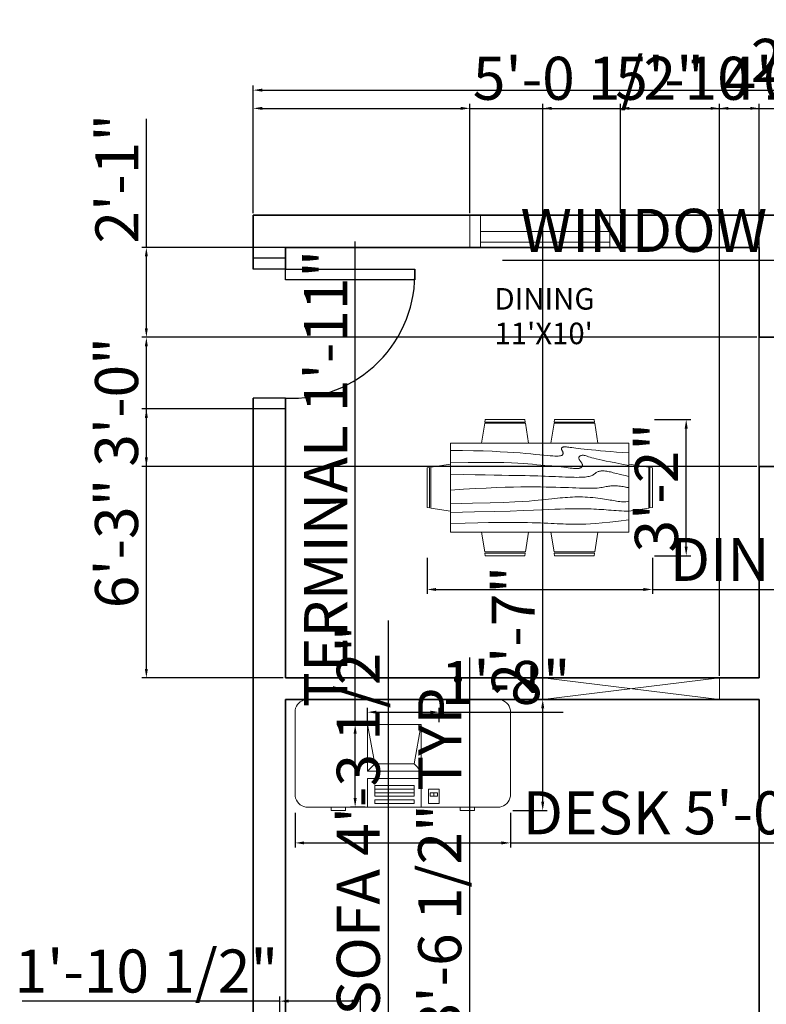
# Model space of a CAD drawing. Units: inches. Extents: x 2011 to 2548, y 530 to 1188.
# Tile 3 of 5: x 2011 to 2220, y 891 to 1166. Entities that reach past the tile are written whole.
import ezdxf

# ---------------------------------------------------------------- set-up
doc = ezdxf.new("R2010")
doc.units = ezdxf.units.IN
for name, color, linetype, lineweight in [('A-ANNO-DIMS', 2, 'Continuous', 18), ('A-AREA-IDEN', 7, 'Continuous', 25), ('A-DOOR', 3, 'Continuous', 25), ('A-EQPM', 8, 'Continuous', 18), ('A-FURN', 8, 'Continuous', 18), ('A-GLAZ', 4, 'Continuous', 18), ('A-WALL', 7, 'Continuous', 35), ('A-WALL-OPEN', 4, 'Continuous', 18)]:
    doc.layers.add(name, color=color, linetype=linetype, lineweight=lineweight)
doc.styles.get("Standard").update_dxf_attribs({"font": 'arial.ttf'})
doc.dimstyles.new('ISO-25', dxfattribs={"dimtxt": 12, "dimasz": 2.5, "dimexe": 1.25, "dimexo": 0.625, "dimtad": 1, "dimdec": 1, "dimlunit": 3, "dimtxsty": 'Standard', "dimcen": 2.5, "dimadec": 0, "dimazin": 0, "dimtfac": 1, "dimtdec": 1, "dimtmove": 0, "dimatfit": 3, "dimfxl": 1, "dimarcsym": 0})

# ---------------------------------------------------------------- blocks, each defined once
blk = doc.blocks.new('Desk - 30 x 60 in.')
for p, q in [((-26.999995, 0), (26.999995, 0)), ((-29.999995, -27), (-29.999995, -3)), ((29.999995, -3), (29.999995, -27)), ((26.999995, -30), (-26.999995, -30)), ((-20.000005, -30), (-20.000005, -31)), ((-16.000005, -31), (-16.000005, -30)), ((15.999995, -31), (15.999995, -30)), ((19.999995, -30), (19.999995, -31)), ((-20.000005, -31), (-16.000005, -31)), ((19.999995, -31), (15.999995, -31))]:
    blk.add_line(p, q)
for centre, start, end in [((-26.499995, -3.5), 98.1301, 171.8699), ((26.499995, -3.5), 8.130102, 81.8699), ((-26.499995, -26.5), 188.1301, 261.8699), ((26.499995, -26.5), 278.1301, 351.8699)]:
    blk.add_arc(centre, 3.535534, start, end)
blk = doc.blocks.new('Computer Terminal')
for p, q in [((-10, 11.5), (5, 11.5)), ((-8, 0.5), (-10, 11.5)), ((-10, -1.5), (-10, 11.5)), ((5, 11.5), (3, 0.5)), ((5, 11.5), (5, -1.5)), ((-10, -1.5), (-8, 0.5)), ((3, 0.5), (-8, 0.5)), ((3, 0.5), (5, -1.5)), ((5, -1.5), (-10, -1.5)), ((-10, -11.5), (-10, -3.5)), ((-10, -3.5), (5, -3.5)), ((5, -3.5), (5, -11.5)), ((-8, -5.5), (-8, -8.5)), ((3, -5.5), (-8, -5.5)), ((3, -6.5), (-8, -6.5)), ((-8, -7.5), (3, -7.5)), ((3, -8.5), (3, -5.5)), ((10, -6.5), (7, -6.5)), ((7, -6.5), (7, -10.5)), ((9.5, -7.5), (7.5, -7.5)), ((7.5, -7.5), (7.5, -8.5)), ((8.5, -7.5), (8.5, -8.5)), ((9.5, -8.5), (9.5, -7.5)), ((10, -10.5), (10, -6.5)), ((-8, -8.5), (3, -8.5)), ((-8, -9.5), (-8, -10.5)), ((3, -9.5), (-8, -9.5)), ((-8, -10.5), (3, -10.5)), ((3, -10.5), (3, -9.5)), ((7, -10.5), (10, -10.5)), ((7.5, -8.5), (9.5, -8.5)), ((5, -11.5), (-10, -11.5))]:
    blk.add_line(p, q)
blk = doc.blocks.new('Dining Set - 36 x 72 in.')
for p, q in [((-22.2343, 26.00059), (-23.4847, 17.99762)), ((-22.2304, 26), (-5.7608, 26)), ((-22, 27.5), (-22.1562, 26.50042)), ((-5.8416, 26.5), (-22.1534, 26.5)), ((-22, 27.5), (-6, 27.5)), ((-5.8437, 26.49966), (-6, 27.5)), ((-4.5152, 17.99762), (-5.7655, 25.99926)), ((5.7657, 26.00059), (4.5153, 17.99762)), ((5.7696, 26), (22.2392, 26)), ((6, 27.5), (5.8438, 26.50042)), ((22.1584, 26.5), (5.8466, 26.5)), ((6, 27.5), (22, 27.5)), ((22.1563, 26.49966), (22, 27.5)), ((23.4848, 17.99762), (22.2345, 25.99926)), ((36, 18), (-36, 18)), ((-36, 18), (-36, -18)), ((36, -18), (36, 18)), ((-45.5, 8), (-44.5004, 8.15617)), ((-45.5, 8), (-45.5, -8)), ((-44.5, -8.15843), (-44.5, 8.15338)), ((-44.0006, 8.23428), (-35.9976, 9.48474)), ((-44, 8.23041), (-44, -8.23915)), ((44.0006, 8.23428), (35.9976, 9.48474)), ((44, 8.23041), (44, -8.23915)), ((44.5, -8.15843), (44.5, 8.15338)), ((45.5, 8), (44.5005, 8.15617)), ((45.5, 8), (45.5, -8)), ((-44.4997, -8.15631), (-45.5, -8)), ((-35.9976, -9.48476), (-43.9993, -8.2345)), ((35.9976, -9.48476), (43.9993, -8.2345)), ((44.4997, -8.15631), (45.5, -8)), ((-36, -18), (36, -18)), ((-22.2343, -26.0006), (-23.4847, -17.99762)), ((-4.5152, -17.99762), (-5.7655, -25.99928)), ((5.7657, -26.0006), (4.5153, -17.99762)), ((23.4848, -17.99762), (22.2345, -25.99928)), ((-22.2304, -26), (-5.7608, -26)), ((-22, -27.5), (-22.1562, -26.50044)), ((-5.8416, -26.5), (-22.1534, -26.5)), ((-22, -27.5), (-6, -27.5)), ((-5.8437, -26.49967), (-6, -27.5)), ((5.7696, -26), (22.2392, -26)), ((6, -27.5), (5.8438, -26.50044)), ((22.1584, -26.5), (5.8466, -26.5)), ((6, -27.5), (22, -27.5)), ((22.1563, -26.49967), (22, -27.5))]:
    blk.add_line(p, q)
for points in [[(-36, 15), (-31.1772, 14.97754), (-26.8079, 14.91406), (-22.8538, 14.81543), (-19.276, 14.6875), (-16.0362, 14.53613), (-13.0957, 14.36718), (-10.4159, 14.18652), (-7.9583, 14), (-5.6904, 13.81315), (-3.6035, 13.63021), (-1.6954, 13.45508), (0.0365, 13.29166), (1.5945, 13.14388), (2.9811, 13.01562), (4.1988, 12.9108), (5.25, 12.83333), (6.1393, 12.78613), (6.8802, 12.76823), (7.4883, 12.77767), (7.9792, 12.8125), (8.3685, 12.87077), (8.6719, 12.95052), (8.9049, 13.0498), (9.0833, 13.16666), (9.2205, 13.29899), (9.3216, 13.44401), (9.3895, 13.59879), (9.4271, 13.76041), (9.4373, 13.92594), (9.4232, 14.09245), (9.3875, 14.257), (9.3333, 14.41666), (9.2638, 14.56917), (9.1836, 14.71484), (9.0975, 14.85465), (9.0104, 14.98958), (8.9272, 15.1206), (8.8529, 15.2487), (8.7922, 15.37483), (8.75, 15.5), (8.7305, 15.62467), (8.7344, 15.74739), (8.7617, 15.86621), (8.8125, 15.97916), (8.8867, 16.08431), (8.9844, 16.17968), (9.1055, 16.26334), (9.25, 16.33333), (9.4189, 16.38802), (9.6172, 16.42708), (9.8506, 16.45052), (10.125, 16.45833), (10.4463, 16.45052), (10.8203, 16.42708), (11.2529, 16.38802), (11.75, 16.33333), (12.3184, 16.26318), (12.9694, 16.17838), (13.7151, 16.07991), (14.5677, 15.96875), (15.5395, 15.84586), (16.6426, 15.71224), (17.8893, 15.56884), (19.2917, 15.41666), (20.859, 15.25667), (22.5879, 15.08984), (24.4721, 14.91715), (26.5052, 14.73958), (28.6809, 14.5581), (30.9929, 14.3737), (33.4347, 14.18733), (36, 14)], [(-36, 10), (-28.9766, 10.14274), (-23.1725, 10.20442), (-18.4241, 10.19775), (-14.5677, 10.13541), (-11.4399, 10.03011), (-8.877, 9.89453), (-6.7154, 9.74137), (-4.7917, 9.58333), (-2.9698, 9.43082), (-1.2246, 9.28515), (0.4415, 9.14534), (2.026, 9.01041), (3.5266, 8.87939), (4.9408, 8.7513), (6.266, 8.62516), (7.5, 8.5), (8.6411, 8.37549), (9.6914, 8.2539), (10.6538, 8.13818), (11.5312, 8.03125), (12.3267, 7.93603), (13.043, 7.85547), (13.6831, 7.79248), (14.25, 7.75), (14.7471, 7.7303), (15.1797, 7.73307), (15.5537, 7.75732), (15.875, 7.80208), (16.1494, 7.86637), (16.3828, 7.94922), (16.5811, 8.04964), (16.75, 8.16666), (16.8944, 8.29915), (17.0143, 8.44531), (17.1089, 8.60319), (17.1771, 8.77083), (17.218, 8.94629), (17.2305, 9.1276), (17.2137, 9.31282), (17.1667, 9.5), (17.0895, 9.6875), (16.987, 9.875), (16.8649, 10.0625), (16.7292, 10.25), (16.5856, 10.4375), (16.4401, 10.625), (16.2985, 10.8125), (16.1667, 11), (16.05, 11.18733), (15.9518, 11.3737), (15.8752, 11.5581), (15.8229, 11.73958), (15.798, 11.91715), (15.8034, 12.08984), (15.842, 12.25667), (15.9167, 12.41666), (16.0295, 12.56836), (16.1784, 12.70833), (16.3605, 12.83268), (16.5729, 12.9375), (16.8127, 13.01888), (17.0768, 13.07291), (17.3625, 13.0957), (17.6667, 13.08333), (17.9894, 13.03312), (18.3418, 12.94726), (18.7382, 12.82918), (19.1927, 12.68229), (19.7195, 12.51001), (20.3327, 12.31575), (21.0465, 12.10294), (21.875, 11.875), (22.8357, 11.63354), (23.959, 11.37304), (25.2786, 11.08618), (26.8282, 10.76562), (28.6414, 10.40405), (30.752, 9.99414), (33.1936, 9.52856), (36, 9)], [(-36, 5.5), (-30.7157, 5.3348), (-26.069, 5.20963), (-21.9946, 5.11767), (-18.4271, 5.05208), (-15.3009, 5.00602), (-12.5508, 4.97265), (-10.1112, 4.94515), (-7.9167, 4.91666), (-5.909, 4.88167), (-4.0586, 4.83984), (-2.3429, 4.79215), (-0.7396, 4.73958), (0.7739, 4.6831), (2.22, 4.6237), (3.6213, 4.56233), (5, 4.5), (6.373, 4.43782), (7.7344, 4.3776), (9.0723, 4.32129), (10.375, 4.27083), (11.6309, 4.22819), (12.8281, 4.19531), (13.9551, 4.17415), (15, 4.16666), (15.954, 4.17448), (16.819, 4.19791), (17.6001, 4.23698), (18.3021, 4.29166), (18.9299, 4.36198), (19.4883, 4.44791), (19.9823, 4.54948), (20.4167, 4.66666), (20.7969, 4.79899), (21.1302, 4.94401), (21.4245, 5.09879), (21.6875, 5.26041), (21.9271, 5.42594), (22.1511, 5.59245), (22.3672, 5.757), (22.5834, 5.91666), (22.8065, 6.06868), (23.0404, 6.21093), (23.2879, 6.34147), (23.5521, 6.45833), (23.8358, 6.55957), (24.142, 6.64323), (24.4735, 6.70735), (24.8334, 6.75), (25.2235, 6.76969), (25.642, 6.76692), (26.0858, 6.74267), (26.5521, 6.69791), (27.0379, 6.63362), (27.5404, 6.55078), (28.0565, 6.45036), (28.5834, 6.33333), (29.1242, 6.19987), (29.7071, 6.04687), (30.3661, 5.87044), (31.1354, 5.66666), (32.0493, 5.43164), (33.142, 5.16146), (34.4475, 4.85221), (36, 4.5)], [(-36, -1), (-30.7915, -0.6591), (-26.0195, -0.38216), (-21.6519, -0.16284), (-17.6563, 0.00521), (-14.0005, 0.12833), (-10.6523, 0.21289), (-7.5796, 0.26522), (-4.75, 0.29166), (-2.134, 0.29793), (0.2878, 0.28711), (2.5317, 0.26163), (4.6146, 0.22396), (6.5529, 0.17651), (8.3633, 0.12174), (10.0623, 0.06209), (11.6667, 0), (13.1899, -0.06201), (14.6341, -0.1211), (15.9982, -0.17432), (17.2813, -0.21875), (18.4823, -0.25147), (19.6003, -0.26953), (20.6343, -0.27002), (21.5834, -0.25), (22.4481, -0.20768), (23.2357, -0.14584), (23.9549, -0.06836), (24.6146, 0.02083), (25.2235, 0.11784), (25.7904, 0.21875), (26.3241, 0.31966), (26.8334, 0.41666), (27.3265, 0.50618), (27.8099, 0.58593), (28.2894, 0.65397), (28.7709, 0.70833), (29.2601, 0.74707), (29.763, 0.76823), (30.2855, 0.76985), (30.8334, 0.75), (31.4088, 0.70784), (31.9994, 0.64713), (32.589, 0.57275), (33.1615, 0.48958), (33.7008, 0.4025), (34.1908, 0.3164), (34.6153, 0.23616), (34.9584, 0.16666), (35.2099, 0.11165), (35.3848, 0.07031), (35.504, 0.04069), (35.5886, 0.02083), (35.6594, 0.00879), (35.7377, 0.0026), (35.8442, 0.00032), (36, 0)], [(-36, -6.5), (-27.1843, -6.31267), (-20.084, -6.1263), (-14.469, -5.9419), (-10.1094, -5.76042), (-6.7752, -5.58285), (-4.2363, -5.41016), (-2.2629, -5.24333), (-0.625, -5.08334), (0.8708, -4.93099), (2.2715, -4.78646), (3.5872, -4.64974), (4.8281, -4.52084), (6.0046, -4.39974), (7.127, -4.28646), (8.2053, -4.18099), (9.25, -4.08334), (10.2705, -3.99382), (11.2734, -3.91407), (12.2647, -3.84603), (13.25, -3.79167), (14.2354, -3.75293), (15.2266, -3.73177), (16.2295, -3.73015), (17.25, -3.75), (18.2912, -3.79248), (19.3451, -3.85547), (20.4009, -3.93604), (21.4479, -4.03125), (22.4754, -4.13819), (23.4727, -4.25391), (24.4289, -4.37549), (25.3334, -4.5), (26.1785, -4.62492), (26.9694, -4.74935), (27.7145, -4.87281), (28.4219, -4.99479), (29.1, -5.11483), (29.7572, -5.23242), (30.4016, -5.34709), (31.0417, -5.45834), (31.6837, -5.56437), (32.3262, -5.65821), (32.9658, -5.73153), (33.599, -5.77604), (34.2224, -5.78345), (34.8327, -5.74545), (35.4264, -5.65373), (36, -5.5)], [(-36, -10), (-26.4022, -9.81299), (-18.4675, -9.62891), (-11.9839, -9.45069), (-6.7396, -9.28125), (-2.5226, -9.12354), (0.8789, -8.98047), (3.6769, -8.85498), (6.0833, -8.75), (8.2767, -8.66765), (10.3021, -8.60677), (12.1712, -8.56543), (13.8958, -8.54167), (15.4876, -8.53353), (16.9583, -8.53907), (18.3197, -8.55632), (19.5834, -8.58334), (20.7616, -8.61841), (21.8685, -8.66081), (22.9188, -8.71004), (23.9271, -8.76563), (24.9081, -8.82707), (25.8763, -8.89388), (26.8465, -8.96558), (27.8334, -9.04167), (28.8474, -9.12118), (29.8828, -9.20117), (30.93, -9.27824), (31.9792, -9.34896), (33.0205, -9.40991), (34.0443, -9.45768), (35.0407, -9.48885), (36, -9.5)], [(-36, -14.5), (-30.0881, -14.33513), (-25.0332, -14.21224), (-20.7312, -14.12647), (-17.0781, -14.07292), (-13.97, -14.04671), (-11.3027, -14.04297), (-8.9724, -14.05681), (-6.875, -14.08334), (-4.9224, -14.11833), (-3.0905, -14.16016), (-1.3709, -14.20785), (0.2448, -14.26042), (1.7647, -14.3169), (3.1973, -14.3763), (4.5507, -14.43767), (5.8333, -14.5), (7.0554, -14.5621), (8.235, -14.62175), (9.3922, -14.67652), (10.5469, -14.72396), (11.7192, -14.76164), (12.929, -14.78711), (14.1965, -14.79794), (15.5417, -14.79167), (16.9933, -14.76424), (18.6152, -14.70508), (20.4804, -14.60197), (22.6615, -14.44271), (25.2312, -14.21509), (28.2624, -13.9069), (31.8277, -13.50594), (36, -13)]]:
    blk.add_lwpolyline(points)
blk = doc.blocks.new('*D12')
at = {"layer": 'A-ANNO-DIMS', "color": 0, "lineweight": -2, "transparency": 16777216}
for p, q in [((2076.53, 1111.98), (2076.53, 1147.49)), ((2079.03, 1146.24), (2374.03, 1146.24)), ((2376.53, 1111.98), (2376.53, 1147.49))]:
    blk.add_line(p, q, dxfattribs=at)
at = {"layer": 'A-ANNO-DIMS', "color": 0, "transparency": 16777216}
for points in [[(2079.03, 1146.66), (2079.03, 1145.82), (2076.53, 1146.24)], [(2374.03, 1146.66), (2374.03, 1145.82), (2376.53, 1146.24)]]:
    blk.add_solid(points, dxfattribs=at)
at = {"layer": 'Defpoints', "color": 0, "transparency": 16777216}
for p in [(2376.53, 1146.24), (2076.53, 1111.36), (2376.53, 1111.36)]:
    blk.add_point(p, dxfattribs=at)
at = {"layer": 'A-ANNO-DIMS', "color": 0, "transparency": 16777216, "insert": (2226.53, 1152.99), "char_height": 12, "attachment_point": 5}
blk.add_mtext("25'", dxfattribs=at)
blk = doc.blocks.new('WIN-36IN')
for p, q in [((0, 42), (9, 42)), ((0, 3), (0, 39)), ((0, 39), (9, 39)), ((1.5, 39), (1.5, 3)), ((4.5, 39), (4.5, 3)), ((9, 39), (9, 3)), ((9, 3), (0, 3)), ((9, 0), (0, 0))]:
    blk.add_line(p, q)
blk = doc.blocks.new('*D19')
at = {"layer": 'A-ANNO-DIMS', "color": 0, "lineweight": -2, "transparency": 16777216}
for p, q in [((2331.36, 1101.73), (2331.36, 1097.51)), ((2355.36, 1101.73), (2355.36, 1097.51)), ((2331.36, 1098.76), (2145.96, 1098.76)), ((2352.86, 1098.76), (2333.86, 1098.76))]:
    blk.add_line(p, q, dxfattribs=at)
at = {"layer": 'A-ANNO-DIMS', "color": 0, "transparency": 16777216}
for points in [[(2333.86, 1099.18), (2333.86, 1098.34), (2331.36, 1098.76)], [(2352.86, 1099.18), (2352.86, 1098.34), (2355.36, 1098.76)]]:
    blk.add_solid(points, dxfattribs=at)
at = {"layer": 'Defpoints', "color": 0, "transparency": 16777216}
for p in [(2331.36, 1102.36), (2355.36, 1102.36), (2331.36, 1098.76)]:
    blk.add_point(p, dxfattribs=at)
at = {"layer": 'A-ANNO-DIMS', "color": 0, "transparency": 16777216, "insert": (2237.41, 1105.59), "char_height": 12, "attachment_point": 5}
blk.add_mtext('WINDOW W2 2\'-0" TYP.', dxfattribs=at)
blk = doc.blocks.new('*D21')
at = {"layer": 'A-ANNO-DIMS', "color": 0, "lineweight": -2, "transparency": 16777216}
for p, q in [((2136.89, 802.78), (2136.89, 988.08)), ((2131.15, 802.78), (2138.14, 802.78)), ((2136.89, 762.86), (2136.89, 800.28)), ((2131.15, 760.36), (2138.14, 760.36))]:
    blk.add_line(p, q, dxfattribs=at)
at = {"layer": 'A-ANNO-DIMS', "color": 0, "transparency": 16777216}
for points in [[(2136.47, 800.28), (2137.31, 800.28), (2136.89, 802.78)], [(2136.47, 762.86), (2137.31, 762.86), (2136.89, 760.36)]]:
    blk.add_solid(points, dxfattribs=at)
at = {"layer": 'Defpoints', "color": 0, "transparency": 16777216}
for p in [(2130.53, 802.78), (2136.89, 802.78), (2130.53, 760.36)]:
    blk.add_point(p, dxfattribs=at)
at = {"layer": 'A-ANNO-DIMS', "color": 0, "transparency": 16777216, "insert": (2130.05, 896.68), "char_height": 12, "attachment_point": 5, "rotation": 90}
blk.add_mtext('DOOR D1 3\'-6 1/2" TYP.', dxfattribs=at)
blk = doc.blocks.new('*D31')
at = {"layer": 'A-ANNO-DIMS', "color": 0, "lineweight": -2, "transparency": 16777216}
for p, q in [((2088.21, 944.73), (2088.21, 935.11)), ((2148.21, 944.73), (2148.21, 935.11)), ((2090.71, 936.36), (2145.71, 936.36)), ((2148.21, 936.36), (2233.57, 936.36))]:
    blk.add_line(p, q, dxfattribs=at)
at = {"layer": 'A-ANNO-DIMS', "color": 0, "transparency": 16777216}
for points in [[(2090.71, 936.78), (2090.71, 935.94), (2088.21, 936.36)], [(2145.71, 936.78), (2145.71, 935.94), (2148.21, 936.36)]]:
    blk.add_solid(points, dxfattribs=at)
at = {"layer": 'Defpoints', "color": 0, "transparency": 16777216}
for p in [(2088.21, 945.36), (2148.21, 945.36), (2148.21, 936.36)]:
    blk.add_point(p, dxfattribs=at)
at = {"layer": 'A-ANNO-DIMS', "color": 0, "transparency": 16777216, "insert": (2192.14, 943.19), "char_height": 12, "attachment_point": 5}
blk.add_mtext('DESK 5\'-0"', dxfattribs=at)
blk = doc.blocks.new('*D32')
at = {"layer": 'A-ANNO-DIMS', "color": 0, "lineweight": -2, "transparency": 16777216}
for p, q in [((2157.21, 976.36), (2157.21, 1012.21)), ((2148.83, 976.36), (2158.46, 976.36)), ((2157.21, 947.86), (2157.21, 973.86)), ((2148.83, 945.36), (2158.46, 945.36))]:
    blk.add_line(p, q, dxfattribs=at)
at = {"layer": 'A-ANNO-DIMS', "color": 0, "transparency": 16777216}
for points in [[(2156.79, 973.86), (2157.63, 973.86), (2157.21, 976.36)], [(2156.79, 947.86), (2157.63, 947.86), (2157.21, 945.36)]]:
    blk.add_solid(points, dxfattribs=at)
at = {"layer": 'Defpoints', "color": 0, "transparency": 16777216}
for p in [(2148.21, 976.36), (2157.21, 976.36), (2148.21, 945.36)]:
    blk.add_point(p, dxfattribs=at)
at = {"layer": 'A-ANNO-DIMS', "color": 0, "transparency": 16777216, "insert": (2150.56, 995.54), "char_height": 12, "attachment_point": 5, "rotation": 90}
blk.add_mtext('2\'-7"', dxfattribs=at)
blk = doc.blocks.new('*D33')
at = {"layer": 'A-ANNO-DIMS', "color": 0, "lineweight": -2, "transparency": 16777216}
for p, q in [((2104.92, 969.36), (2104.92, 1104.05)), ((2107.74, 969.36), (2103.67, 969.36)), ((2104.92, 948.86), (2104.92, 966.86)), ((2107.74, 946.36), (2103.67, 946.36))]:
    blk.add_line(p, q, dxfattribs=at)
at = {"layer": 'A-ANNO-DIMS', "color": 0, "transparency": 16777216}
for points in [[(2104.5, 966.86), (2105.34, 966.86), (2104.92, 969.36)], [(2104.5, 948.86), (2105.34, 948.86), (2104.92, 946.36)]]:
    blk.add_solid(points, dxfattribs=at)
at = {"layer": 'Defpoints', "color": 0, "transparency": 16777216}
for p in [(2104.92, 969.36), (2108.37, 969.36), (2108.37, 946.36)]:
    blk.add_point(p, dxfattribs=at)
at = {"layer": 'A-ANNO-DIMS', "color": 0, "transparency": 16777216, "insert": (2098.26, 1037.96), "char_height": 12, "attachment_point": 5, "rotation": 90}
blk.add_mtext('TERMINAL 1\'-11"', dxfattribs=at)
blk = doc.blocks.new('*D34')
at = {"layer": 'A-ANNO-DIMS', "color": 0, "lineweight": -2, "transparency": 16777216}
for p, q in [((2108.37, 969.98), (2108.37, 974.06)), ((2110.87, 972.81), (2125.87, 972.81)), ((2128.37, 969.98), (2128.37, 974.06)), ((2128.37, 972.81), (2162.89, 972.81))]:
    blk.add_line(p, q, dxfattribs=at)
at = {"layer": 'A-ANNO-DIMS', "color": 0, "transparency": 16777216}
for points in [[(2110.87, 973.23), (2110.87, 972.39), (2108.37, 972.81)], [(2125.87, 973.23), (2125.87, 972.39), (2128.37, 972.81)]]:
    blk.add_solid(points, dxfattribs=at)
at = {"layer": 'Defpoints', "color": 0, "transparency": 16777216}
for p in [(2128.37, 972.81), (2108.37, 969.36), (2128.37, 969.36)]:
    blk.add_point(p, dxfattribs=at)
at = {"layer": 'A-ANNO-DIMS', "color": 0, "transparency": 16777216, "insert": (2146.88, 979.56), "char_height": 12, "attachment_point": 5}
blk.add_mtext('1\'-8"', dxfattribs=at)
blk = doc.blocks.new('*D35')
at = {"layer": 'A-ANNO-DIMS', "color": 0, "lineweight": -2, "transparency": 16777216}
for p, q in [((2124.99, 1015.81), (2124.99, 1005.77)), ((2187.78, 1015.81), (2187.78, 1005.77)), ((2127.49, 1007.02), (2185.28, 1007.02)), ((2187.78, 1007.02), (2323.42, 1007.02))]:
    blk.add_line(p, q, dxfattribs=at)
at = {"layer": 'A-ANNO-DIMS', "color": 0, "transparency": 16777216}
for points in [[(2127.49, 1007.44), (2127.49, 1006.6), (2124.99, 1007.02)], [(2185.28, 1007.44), (2185.28, 1006.6), (2187.78, 1007.02)]]:
    blk.add_solid(points, dxfattribs=at)
at = {"layer": 'Defpoints', "color": 0, "transparency": 16777216}
for p in [(2124.99, 1016.44), (2187.78, 1016.44), (2187.78, 1007.02)]:
    blk.add_point(p, dxfattribs=at)
at = {"layer": 'A-ANNO-DIMS', "color": 0, "transparency": 16777216, "insert": (2256.85, 1013.85), "char_height": 12, "attachment_point": 5}
blk.add_mtext('DINING SET 5\'-3"', dxfattribs=at)
blk = doc.blocks.new('*D36')
at = {"layer": 'A-ANNO-DIMS', "color": 0, "lineweight": -2, "transparency": 16777216}
for p, q in [((2188.4, 1054.39), (2198.45, 1054.39)), ((2197.2, 1018.94), (2197.2, 1051.89)), ((2188.4, 1016.44), (2198.45, 1016.44))]:
    blk.add_line(p, q, dxfattribs=at)
at = {"layer": 'A-ANNO-DIMS', "color": 0, "transparency": 16777216}
for points in [[(2196.78, 1051.89), (2197.61, 1051.89), (2197.2, 1054.39)], [(2196.78, 1018.94), (2197.61, 1018.94), (2197.2, 1016.44)]]:
    blk.add_solid(points, dxfattribs=at)
at = {"layer": 'Defpoints', "color": 0, "transparency": 16777216}
for p in [(2187.78, 1054.39), (2197.2, 1054.39), (2187.78, 1016.44)]:
    blk.add_point(p, dxfattribs=at)
at = {"layer": 'A-ANNO-DIMS', "color": 0, "transparency": 16777216, "insert": (2190.44, 1035.41), "char_height": 12, "attachment_point": 5, "rotation": 90}
blk.add_mtext('3\'-2"', dxfattribs=at)
blk = doc.blocks.new('*D37')
at = {"layer": 'A-ANNO-DIMS', "color": 0, "lineweight": -2, "transparency": 16777216}
for p, q in [((2114.19, 884.5), (2114.19, 998.36)), ((2107.06, 884.5), (2115.44, 884.5)), ((2114.19, 835.34), (2114.19, 882)), ((2107.06, 832.84), (2115.44, 832.84))]:
    blk.add_line(p, q, dxfattribs=at)
at = {"layer": 'A-ANNO-DIMS', "color": 0, "transparency": 16777216}
for points in [[(2113.77, 882), (2114.61, 882), (2114.19, 884.5)], [(2113.77, 835.34), (2114.61, 835.34), (2114.19, 832.84)]]:
    blk.add_solid(points, dxfattribs=at)
at = {"layer": 'Defpoints', "color": 0, "transparency": 16777216}
for p in [(2106.44, 884.5), (2114.19, 884.5), (2106.44, 832.84)]:
    blk.add_point(p, dxfattribs=at)
at = {"layer": 'A-ANNO-DIMS', "color": 0, "transparency": 16777216, "insert": (2107.35, 942.68), "char_height": 12, "attachment_point": 5, "rotation": 90}
blk.add_mtext('SOFA 4\'-3 1/2"', dxfattribs=at)
blk = doc.blocks.new('*D38')
at = {"layer": 'A-ANNO-DIMS', "color": 0, "lineweight": -2, "transparency": 16777216}
for p, q in [((2083.89, 892.25), (2012.08, 892.25)), ((2083.89, 885.13), (2083.89, 893.5)), ((2103.94, 892.25), (2086.39, 892.25)), ((2106.44, 885.13), (2106.44, 893.5))]:
    blk.add_line(p, q, dxfattribs=at)
at = {"layer": 'A-ANNO-DIMS', "color": 0, "transparency": 16777216}
for points in [[(2086.39, 892.67), (2086.39, 891.84), (2083.89, 892.25)], [(2103.94, 892.67), (2103.94, 891.84), (2106.44, 892.25)]]:
    blk.add_solid(points, dxfattribs=at)
at = {"layer": 'Defpoints', "color": 0, "transparency": 16777216}
for p in [(2083.89, 892.25), (2083.89, 884.5), (2106.44, 884.5)]:
    blk.add_point(p, dxfattribs=at)
at = {"layer": 'A-ANNO-DIMS', "color": 0, "transparency": 16777216, "insert": (2046.73, 899.08), "char_height": 12, "attachment_point": 5}
blk.add_mtext('1\'-10 1/2"', dxfattribs=at)
blk = doc.blocks.new('*D47')
at = {"layer": 'A-ANNO-DIMS', "color": 0, "lineweight": -2, "transparency": 16777216}
for p, q in [((2076.53, 1111.98), (2076.53, 1142.41)), ((2136.88, 1111.98), (2136.88, 1142.41)), ((2079.03, 1141.16), (2134.38, 1141.16)), ((2136.88, 1141.16), (2200.49, 1141.16))]:
    blk.add_line(p, q, dxfattribs=at)
at = {"layer": 'A-ANNO-DIMS', "color": 0, "transparency": 16777216}
for points in [[(2079.03, 1141.58), (2079.03, 1140.74), (2076.53, 1141.16)], [(2134.38, 1141.58), (2134.38, 1140.74), (2136.88, 1141.16)]]:
    blk.add_solid(points, dxfattribs=at)
at = {"layer": 'Defpoints', "color": 0, "transparency": 16777216}
for p in [(2136.88, 1141.16), (2076.53, 1111.36), (2136.88, 1111.36)]:
    blk.add_point(p, dxfattribs=at)
at = {"layer": 'A-ANNO-DIMS', "color": 0, "transparency": 16777216, "insert": (2169.94, 1147.99), "char_height": 12, "attachment_point": 5}
blk.add_mtext('5\'-0 1/2"', dxfattribs=at)
blk = doc.blocks.new('*D48')
at = {"layer": 'A-ANNO-DIMS', "color": 0, "lineweight": -2, "transparency": 16777216}
for p, q in [((2178.88, 1111.98), (2178.88, 1142.41)), ((2249.46, 1111.98), (2249.46, 1142.41)), ((2181.38, 1141.16), (2246.96, 1141.16))]:
    blk.add_line(p, q, dxfattribs=at)
at = {"layer": 'A-ANNO-DIMS', "color": 0, "transparency": 16777216}
for points in [[(2181.38, 1141.58), (2181.38, 1140.74), (2178.88, 1141.16)], [(2246.96, 1141.58), (2246.96, 1140.74), (2249.46, 1141.16)]]:
    blk.add_solid(points, dxfattribs=at)
at = {"layer": 'Defpoints', "color": 0, "transparency": 16777216}
for p in [(2249.46, 1141.16), (2178.88, 1111.36), (2249.46, 1111.36)]:
    blk.add_point(p, dxfattribs=at)
at = {"layer": 'A-ANNO-DIMS', "color": 0, "transparency": 16777216, "insert": (2214.17, 1147.99), "char_height": 12, "attachment_point": 5}
blk.add_mtext('5\'-10 1/2"', dxfattribs=at)
blk = doc.blocks.new('*D54')
at = {"layer": 'A-ANNO-DIMS', "color": 0, "lineweight": -2, "transparency": 16777216}
for p, q in [((2223.53, 891.73), (2223.53, 540.31)), ((2217.53, 885.73), (2217.53, 540.31)), ((2215.03, 541.56), (2212.53, 541.56)), ((2217.53, 541.56), (2223.53, 541.56)), ((2226.03, 541.56), (2261.68, 541.56))]:
    blk.add_line(p, q, dxfattribs=at)
at = {"layer": 'A-ANNO-DIMS', "color": 0, "transparency": 16777216}
for points in [[(2215.03, 541.98), (2215.03, 541.14), (2217.53, 541.56)], [(2226.03, 541.98), (2226.03, 541.14), (2223.53, 541.56)]]:
    blk.add_solid(points, dxfattribs=at)
at = {"layer": 'Defpoints', "color": 0, "transparency": 16777216}
for p in [(2223.53, 892.36), (2217.53, 886.36), (2223.53, 541.56)]:
    blk.add_point(p, dxfattribs=at)
at = {"layer": 'A-ANNO-DIMS', "color": 0, "transparency": 16777216, "insert": (2245.1, 548.31), "char_height": 12, "attachment_point": 5}
blk.add_mtext('0\'-6"', dxfattribs=at)
blk = doc.blocks.new('*D55')
at = {"layer": 'A-ANNO-DIMS', "color": 0, "lineweight": -2, "transparency": 16777216}
for p, q in [((2216.9, 1077.32), (2045.48, 1077.32)), ((2046.73, 1043.82), (2046.73, 1074.82)), ((2216.9, 1041.32), (2045.48, 1041.32))]:
    blk.add_line(p, q, dxfattribs=at)
at = {"layer": 'A-ANNO-DIMS', "color": 0, "transparency": 16777216}
for points in [[(2046.31, 1074.82), (2047.14, 1074.82), (2046.73, 1077.32)], [(2046.31, 1043.82), (2047.14, 1043.82), (2046.73, 1041.32)]]:
    blk.add_solid(points, dxfattribs=at)
at = {"layer": 'Defpoints', "color": 0, "transparency": 16777216}
for p in [(2046.73, 1077.32), (2217.53, 1077.32), (2217.53, 1041.32)]:
    blk.add_point(p, dxfattribs=at)
at = {"layer": 'A-ANNO-DIMS', "color": 0, "transparency": 16777216, "insert": (2039.97, 1059.32), "char_height": 12, "attachment_point": 5, "rotation": 90}
blk.add_mtext('3\'-0"', dxfattribs=at)
blk = doc.blocks.new('*D56')
at = {"layer": 'A-ANNO-DIMS', "color": 0, "lineweight": -2, "transparency": 16777216}
for p, q in [((2046.73, 1102.36), (2046.73, 1138.21)), ((2216.9, 1102.36), (2045.48, 1102.36)), ((2046.73, 1079.82), (2046.73, 1099.86)), ((2216.9, 1077.32), (2045.48, 1077.32))]:
    blk.add_line(p, q, dxfattribs=at)
at = {"layer": 'A-ANNO-DIMS', "color": 0, "transparency": 16777216}
for points in [[(2046.31, 1099.86), (2047.14, 1099.86), (2046.73, 1102.36)], [(2046.31, 1079.82), (2047.14, 1079.82), (2046.73, 1077.32)]]:
    blk.add_solid(points, dxfattribs=at)
at = {"layer": 'Defpoints', "color": 0, "transparency": 16777216}
for p in [(2046.73, 1102.36), (2217.53, 1102.36), (2217.53, 1077.32)]:
    blk.add_point(p, dxfattribs=at)
at = {"layer": 'A-ANNO-DIMS', "color": 0, "transparency": 16777216, "insert": (2040.08, 1121.54), "char_height": 12, "attachment_point": 5, "rotation": 90}
blk.add_mtext('2\'-1"', dxfattribs=at)
blk = doc.blocks.new('*D58')
at = {"layer": 'A-ANNO-DIMS', "color": 0, "lineweight": -2, "transparency": 16777216}
for p, q in [((2157.2, 982.98), (2157.2, 1142.41)), ((2206.48, 982.98), (2206.48, 1142.41)), ((2159.7, 1141.16), (2203.98, 1141.16)), ((2206.48, 1141.16), (2270.57, 1141.16))]:
    blk.add_line(p, q, dxfattribs=at)
at = {"layer": 'A-ANNO-DIMS', "color": 0, "transparency": 16777216}
for points in [[(2159.7, 1141.58), (2159.7, 1140.74), (2157.2, 1141.16)], [(2203.98, 1141.58), (2203.98, 1140.74), (2206.48, 1141.16)]]:
    blk.add_solid(points, dxfattribs=at)
at = {"layer": 'Defpoints', "color": 0, "transparency": 16777216}
for p in [(2206.48, 1141.16), (2157.2, 982.36), (2206.48, 982.36)]:
    blk.add_point(p, dxfattribs=at)
at = {"layer": 'A-ANNO-DIMS', "color": 0, "transparency": 16777216, "insert": (2239.78, 1147.99), "char_height": 12, "attachment_point": 5}
blk.add_mtext('4\'-1 1/2"', dxfattribs=at)
blk = doc.blocks.new('*D59')
at = {"layer": 'A-ANNO-DIMS', "color": 0, "lineweight": -2, "transparency": 16777216}
for p, q in [((2206.48, 982.98), (2206.48, 1142.41)), ((2217.53, 982.98), (2217.53, 1142.41)), ((2208.98, 1141.16), (2215.03, 1141.16)), ((2217.53, 1141.16), (2262.5, 1141.16))]:
    blk.add_line(p, q, dxfattribs=at)
at = {"layer": 'A-ANNO-DIMS', "color": 0, "transparency": 16777216}
for points in [[(2208.98, 1141.58), (2208.98, 1140.74), (2206.48, 1141.16)], [(2215.03, 1141.58), (2215.03, 1140.74), (2217.53, 1141.16)]]:
    blk.add_solid(points, dxfattribs=at)
at = {"layer": 'Defpoints', "color": 0, "transparency": 16777216}
for p in [(2217.53, 1141.16), (2206.48, 982.36), (2217.53, 982.36)]:
    blk.add_point(p, dxfattribs=at)
at = {"layer": 'A-ANNO-DIMS', "color": 0, "transparency": 16777216, "insert": (2241.26, 1147.91), "char_height": 12, "attachment_point": 5}
blk.add_mtext('0\'-11"', dxfattribs=at)
blk = doc.blocks.new('*D62')
at = {"layer": 'A-ANNO-DIMS', "color": 0, "lineweight": -2, "transparency": 16777216}
for p, q in [((2084.9, 1057.36), (2045.48, 1057.36)), ((2046.73, 984.86), (2046.73, 1054.86)), ((2084.9, 982.36), (2045.48, 982.36))]:
    blk.add_line(p, q, dxfattribs=at)
at = {"layer": 'A-ANNO-DIMS', "color": 0, "transparency": 16777216}
for points in [[(2046.31, 1054.86), (2047.14, 1054.86), (2046.73, 1057.36)], [(2046.31, 984.86), (2047.14, 984.86), (2046.73, 982.36)]]:
    blk.add_solid(points, dxfattribs=at)
at = {"layer": 'Defpoints', "color": 0, "transparency": 16777216}
for p in [(2046.73, 1057.36), (2085.53, 1057.36), (2085.53, 982.36)]:
    blk.add_point(p, dxfattribs=at)
at = {"layer": 'A-ANNO-DIMS', "color": 0, "transparency": 16777216, "insert": (2039.97, 1019.86), "char_height": 12, "attachment_point": 5, "rotation": 90}
blk.add_mtext('6\'-3"', dxfattribs=at)

msp = doc.modelspace()

# ---------------------------------------------------------------- linework, layer by layer
at = {"layer": 'A-DOOR'}
for p, q in [((2085.53, 1099.36), (2076.53, 1099.36)), ((2085.53, 1096.36), (2076.53, 1096.36)), ((2085.53, 1060.36), (2076.53, 1060.36)), ((2085.53, 1057.36), (2076.53, 1057.36))]:
    msp.add_line(p, q, dxfattribs=at)
msp.add_lwpolyline([(2085.53, 1096.36), (2121.53, 1096.36), (2121.53, 1093.36), (2085.53, 1093.36)], close=True, dxfattribs=at)
msp.add_arc((2087.03, 1094.86), 34.53, 267.5104, 2.4896, dxfattribs=at)
at = {"layer": 'A-WALL'}
for p, q in [((2085.53, 1102.36), (2085.53, 1096.36)), ((2217.53, 1102.36), (2085.53, 1102.36)), ((2217.53, 1102.36), (2217.53, 1077.32)), ((2217.53, 1077.32), (2223.53, 1077.32)), ((2085.53, 1060.36), (2085.53, 982.36)), ((2217.53, 1041.32), (2223.53, 1041.32)), ((2217.53, 1041.32), (2217.53, 982.36)), ((2217.53, 982.36), (2085.53, 982.36)), ((2217.53, 976.36), (2085.53, 976.36)), ((2085.53, 976.36), (2085.53, 766.36)), ((2217.53, 976.36), (2217.53, 886.36))]:
    msp.add_line(p, q, dxfattribs=at)
msp.add_lwpolyline([(2076.53, 1060.36), (2076.53, 571.36), (2376.53, 571.36), (2376.53, 1111.36), (2076.53, 1111.36), (2076.53, 1096.36)], dxfattribs=at)
at = {"layer": 'A-WALL-OPEN'}
for p, q in [((2157.2, 982.36), (2157.2, 976.36)), ((2157.2, 982.36), (2206.48, 976.36)), ((2157.2, 976.36), (2206.48, 982.36)), ((2206.48, 982.36), (2206.48, 976.36))]:
    msp.add_line(p, q, dxfattribs=at)

# ---------------------------------------------------------------- block references
at = {"layer": 'A-EQPM'}
msp.add_blockref('Computer Terminal', (2118.37, 957.86), dxfattribs=at)
at = {"layer": 'A-FURN', "xscale": 0.690025592957486, "yscale": 0.690025592957486, "zscale": 0.690025592957486}
msp.add_blockref('Dining Set - 36 x 72 in.', (2156.38, 1035.41), dxfattribs=at)
at = {"layer": 'A-FURN'}
msp.add_blockref('Desk - 30 x 60 in.', (2118.21, 976.36), dxfattribs=at)
at = {"layer": 'A-GLAZ', "rotation": 90.00000000000067}
msp.add_blockref('WIN-36IN', (2178.88, 1102.36), dxfattribs=at)

# ---------------------------------------------------------------- texts
at = {"layer": 'A-AREA-IDEN'}
for s, p in [('DINING', (2143.76, 1085.05)), ("11'X10'", (2143.76, 1075.41))]:
    msp.add_text(s, height=6, dxfattribs=at).set_placement(p)

# ---------------------------------------------------------------- dimensions: what is measured, and where the dimension line sits
at = {"layer": 'A-ANNO-DIMS'}
for base, p1, p2, override, picture, middle in [((2136.8828, 1141.1587), (2076.527, 1111.3587), (2136.8828, 1111.3587), {"dimdec": 1, "dimlfac": 1, "dimrnd": 0, "dimzin": 1, "dimdsep": 46, "dimlunit": 4, "dimfrac": 2}, '*D47', (2169.9382, 1147.9883)), ((2206.48, 1141.16), (2157.2, 982.36), (2206.48, 982.36), {"dimdec": 1, "dimlfac": 1, "dimrnd": 0, "dimzin": 1, "dimdsep": 46, "dimlunit": 4, "dimfrac": 2}, '*D58', (2239.78, 1147.99)), ((2249.46, 1141.16), (2178.88, 1111.36), (2249.46, 1111.36), {"dimdec": 1, "dimlfac": 1, "dimrnd": 0, "dimzin": 1, "dimdsep": 46, "dimlunit": 4, "dimfrac": 2}, '*D48', (2214.17, 1147.99)), ((2376.53, 1146.24), (2076.53, 1111.36), (2376.53, 1111.36), {"dimclrd": 0, "dimclre": 0, "dimclrt": 0}, '*D12', (2226.53, 1152.99)), ((2217.527, 1141.1587), (2206.4794, 982.3587), (2217.527, 982.3587), {"dimdec": 1, "dimlfac": 1, "dimrnd": 0, "dimzin": 1, "dimdsep": 46, "dimlunit": 4, "dimfrac": 2}, '*D59', (2241.2632, 1147.9106)), ((2128.37, 972.81), (2108.37, 969.36), (2128.37, 969.36), {"dimdec": 1, "dimlfac": 1, "dimrnd": 0, "dimzin": 1, "dimdsep": 46, "dimlunit": 4, "dimfrac": 2}, '*D34', (2146.88, 979.56)), ((2223.53, 541.56), (2217.53, 886.36), (2223.53, 892.36), {"dimdec": 1, "dimlfac": 1, "dimrnd": 0, "dimzin": 1, "dimdsep": 46, "dimlunit": 4, "dimfrac": 2}, '*D54', (2245.1, 548.31))]:
    dim = msp.add_linear_dim(base=base, p1=p1, p2=p2, dimstyle='ISO-25', override=override, dxfattribs=at)
    dim.commit()
    dim.dimension.update_dxf_attribs({"geometry": picture, "text_midpoint": middle})
for base, p1, p2, angle, text, picture, middle in [((2331.36, 1098.76), (2355.36, 1102.36), (2331.36, 1102.36), 180, 'WINDOW W2 <> TYP.', '*D19', (2237.41, 1105.59)), ((2104.92, 969.36), (2108.37, 946.36), (2108.37, 969.36), 90, 'TERMINAL <>', '*D33', (2098.26, 1037.96)), ((2114.19, 884.5), (2106.44, 832.84), (2106.44, 884.5), 90, 'SOFA <>', '*D37', (2107.35, 942.68)), ((2136.89, 802.78), (2130.53, 760.36), (2130.53, 802.78), 90, 'DOOR D1 <> TYP.', '*D21', (2130.05, 896.68))]:
    dim = msp.add_linear_dim(base=base, p1=p1, p2=p2, angle=angle, text=text, dimstyle='ISO-25', override={"dimdec": 1, "dimlfac": 1, "dimrnd": 0, "dimzin": 1, "dimdsep": 46, "dimlunit": 4, "dimfrac": 2}, dxfattribs=at)
    dim.commit()
    dim.dimension.update_dxf_attribs({"geometry": picture, "text_midpoint": middle})
for base, p1, p2, angle, picture, middle in [((2046.73, 1102.36), (2217.53, 1077.32), (2217.53, 1102.36), 90, '*D56', (2040.08, 1121.54)), ((2046.73, 1077.32), (2217.53, 1041.32), (2217.53, 1077.32), 90, '*D55', (2039.97, 1059.32)), ((2046.73, 1057.36), (2085.53, 982.36), (2085.53, 1057.36), 90, '*D62', (2039.97, 1019.86)), ((2197.1962, 1054.3906), (2187.7774, 1016.4391), (2187.7774, 1054.3906), 90, '*D36', (2190.4402, 1035.4148)), ((2157.21, 976.36), (2148.21, 945.36), (2148.21, 976.36), 90, '*D32', (2150.56, 995.54)), ((2083.8868, 892.2546), (2106.4394, 884.5047), (2083.8868, 884.5047), 180, '*D38', (2046.7345, 899.0843))]:
    dim = msp.add_linear_dim(base=base, p1=p1, p2=p2, angle=angle, dimstyle='ISO-25', override={"dimdec": 1, "dimlfac": 1, "dimrnd": 0, "dimzin": 1, "dimdsep": 46, "dimlunit": 4, "dimfrac": 2}, dxfattribs=at)
    dim.commit()
    dim.dimension.update_dxf_attribs({"geometry": picture, "text_midpoint": middle})
for base, p1, p2, text, picture, middle in [((2187.78, 1007.02), (2124.99, 1016.44), (2187.78, 1016.44), 'DINING SET <>', '*D35', (2256.85, 1013.85)), ((2148.21, 936.36), (2088.21, 945.36), (2148.21, 945.36), 'DESK <>', '*D31', (2192.14, 943.19))]:
    dim = msp.add_linear_dim(base=base, p1=p1, p2=p2, text=text, dimstyle='ISO-25', override={"dimdec": 1, "dimlfac": 1, "dimrnd": 0, "dimzin": 1, "dimdsep": 46, "dimlunit": 4, "dimfrac": 2}, dxfattribs=at)
    dim.commit()
    dim.dimension.update_dxf_attribs({"geometry": picture, "text_midpoint": middle})

doc.saveas('drawing.dxf')
